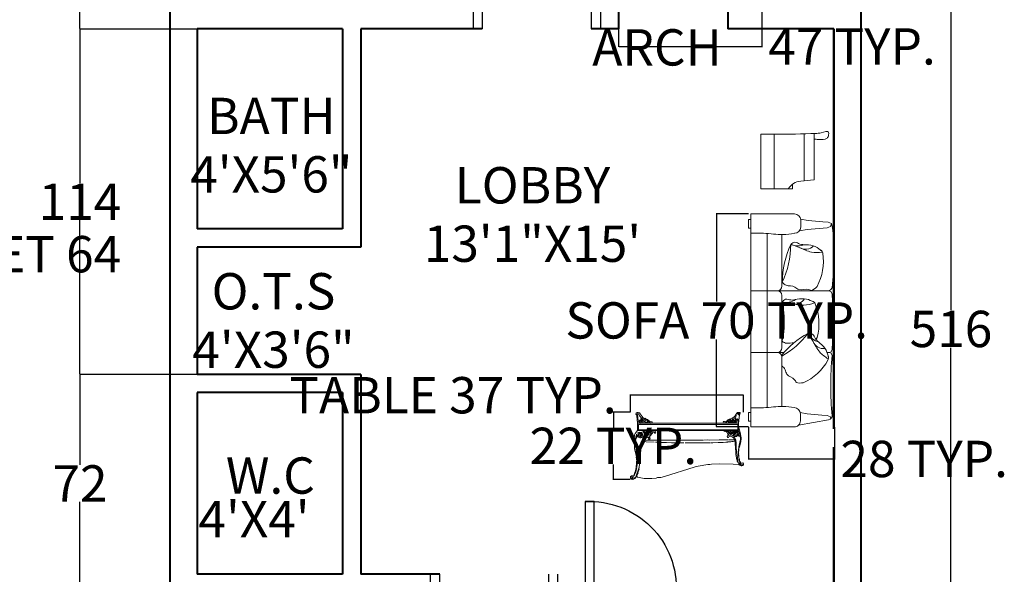
# Model space of a CAD drawing. Units: inches. Extents: x -124 to 612, y -69 to 524.
# Tile 8 of 9: x 287 to 612, y 146 to 329. Entities that reach past the tile are written whole.
import ezdxf
from ezdxf.enums import TextEntityAlignment as Align

# ---------------------------------------------------------------- set-up
doc = ezdxf.new("R2010")
doc.units = ezdxf.units.IN
doc.header["$MEASUREMENT"] = 0
for name, color, linetype, lineweight in [('A-ANNO-DIMS', 2, 'Continuous', 18), ('A-ANNO-TEXT', 1, 'Continuous', 18), ('A-AREA-IDEN', 1, 'Continuous', 18), ('A-DOOR', 4, 'Continuous', 25), ('A-FURN', 8, 'Continuous', 18), ('A-WALL', 7, 'Continuous', 40)]:
    doc.layers.add(name, color=color, linetype=linetype, lineweight=lineweight)
doc.styles.get("Standard").update_dxf_attribs({"font": 'arial.ttf'})
doc.dimstyles.get("Standard").update_dxf_attribs({"dimtxt": 12, "dimasz": 0.18, "dimexe": 0.18, "dimexo": 0.0625, "dimgap": 0.09, "dimtad": 0, "dimtih": 1, "dimtoh": 1, "dimdec": 0, "dimzin": 0, "dimdsep": 46, "dimlunit": 4, "dimtxsty": 'Standard', "dimcen": 0.09, "dimadec": 0, "dimazin": 0, "dimtfac": 1, "dimtdec": 0, "dimtofl": 0, "dimtmove": 0, "dimatfit": 3, "dimfxl": 1, "dimtolj": 1, "dimtzin": 0, "dimarcsym": 0})

# ---------------------------------------------------------------- blocks, each defined once
blk = doc.blocks.new('A$C32C86113')
for p, q in [((77.9, 721.3, -9.2), (82, 773.3, -9.2)), ((82, 773.3, -9.2), (93.6, 803.8, -9.2)), ((93.6, 803.8, -9.2), (123, 812.9, -9.2)), ((736.9, 798.3, -9.2), (719.4, 811.4, -9.2)), ((747.8, 782.5, -9.2), (736.9, 798.3, -9.2)), ((747.6, 163.7, -9.2), (747.6, 782.8, -9.2)), ((747.7, 782.8, -9.2), (758.8, 802, -9.2)), ((758.8, 802, -9.2), (780.7, 812.4, -9.2)), ((1340.4, 800.9, -9.2), (1318.5, 811.4, -9.2)), ((1347.6, 787, -9.2), (1340.4, 800.9, -9.2)), ((1347.6, 787, -9.2), (1354.9, 800.9, -9.2)), ((1347.6, 787, -9.2), (1347.6, 761.5, -9.2)), ((1354.9, 800.9, -9.2), (1376.9, 811.5, -9.2)), ((2056, 484.9, -9.2), (2002, 776.1, -9.2)), ((65.8, 577.5, -9.2), (77.9, 721.3, -9.2)), ((51.2, 502.4, -9.2), (65.8, 577.5, -9.2)), ((60.2, 506.2, -9.2), (128.9, 506.2, -9.2)), ((2013.7, 502.6, -9.2), (1944.9, 502.8, -9.2)), ((0.2, 446.2, -9.2), (0, 20, -9.2)), ((2071.8, 20, 333.6), (2071.8, 442.4, 333.6)), ((702.6, 323.7, -9.2), (200, 323.4, -0.7)), ((1302.6, 323.7, -9.2), (792.6, 323.7, -9.2)), ((1347.6, 343.7, -9.2), (1347.6, 278.7, -9.2)), ((1872.8, 323.7, -9.2), (1392.6, 323.7, -9.2)), ((747.6, 20, -9.2), (747.6, 278.7, -9.2)), ((1347.6, 278.7, -9.2), (1347.6, 20, -9.2)), ((2071.8, 20, 333.6), (0, 20, -9.2)), ((55.9, 20), (55.9, 0)), ((139, 0), (139, 20, 13.8)), ((1932.8, 0), (1932.8, 20, 13.8)), ((2015.9, 20), (2015.9, 0)), ((55.9, 0), (139, 0)), ((2015.9, 0), (1932.8, 0))]:
    blk.add_line(p, q)
at = {"ltscale": 3}
for p, q in [((123, 794.8, -9.2), (93.6, 803.8, -9.2)), ((134.6, 764.2, -9.2), (123, 794.8, -9.2)), ((1960.7, 764.2, -9.2), (1972.3, 794.8, -9.2)), ((1972.3, 794.8, -9.2), (1989.3, 800, -9.2)), ((150.8, 568.4, -9.2), (134.6, 764.2, -9.2)), ((1944.5, 568.4, -9.2), (1956.6, 712.2, -9.2)), ((1956.6, 712.2, -9.2), (1960.7, 764.2, -9.2)), ((165.4, 493.4, -9.2), (150.8, 568.4, -9.2)), ((1931.4, 501.4, -9.2), (1944.5, 568.4, -9.2)), ((191.4, 179.1, 242), (1883, 179.1, 242))]:
    blk.add_line(p, q, dxfattribs=at)
for centre, radius, start, end in [((414.4, -1890.5, -9.2), 2719, 83.56046, 96.1533), ((1675, -2302.2, -9.2), 3127.9, 84.6632, 95.46976), ((1399.9, 730.9, 333.6), 45, 61.39238, 113.21883), ((1178.3, 324.5, 333.6), 507.8, 23.79865, 61.39238), ((1957.7, 767.9, -9.2), 45, 10.50914, 90), ((390.8, 676.1, 333.6), 45, 98.91064, 150.73708), ((462.5, 218.9, 333.6), 507.8, 61.3169, 98.91064), ((1065.4, 175.7, 333.6), 507.8, 74.38291, 111.97665), ((594.5, 543.8, 333.6), 164.4, 23.69861, 47.17942), ((892.1, 605, 333.6), 45, 111.97665, 163.80309), ((1917, 985.8, 333.6), 858.1, 208.49339, 231.11555), ((1120.5, 522.1, 333.6), 164.4, 52.76952, 60.24543), ((60.2, 446.2, -9.2), 60, 90, 179.98162), ((128.9, 446.2, -9.2), 60, 0, 90), ((1480.8, 501.9, 333.6), 164.4, 346.18035, 9.66116), ((1944.7, 442.8, -9.2), 60, 89.78593, 179.78593), ((2014.6, 445.3, 333.6), 57.3, 357.05812, 90.92062), ((691.5, 1297, 333.6), 971.5, 246.03307, 268.4688), ((702.6, 278.7, -9.2), 45, 0, 90), ((792.6, 278.7, -9.2), 45, 90, 180), ((1054.6, -512.3, 333.6), 858.1, 76.95935, 103.04065), ((1302.6, 278.7, -9.2), 45, 0, 90), ((1392.6, 278.7, -9.2), 45, 90, 180)]:
    blk.add_arc(centre, radius, start, end)
for centre, radius, start, end in [((1034.7, -7187.9, -9.2), 8004.3, 87.96784, 91.81809), ((1675, 3925.1, -9.2), 3127.9, 264.53024, 275.3368), ((1072.8, 736, 333.6), 183.2, 299.4203, 342.7126), ((1202.4, 727.4, 333.6), 108.4, 291.46137, 8.04974), ((236.2, 553.1, 333.6), 108.4, 328.97962, 45.56799), ((639.9, -104, 333.6), 858.1, 29.83423, 52.45639), ((128.3, 481, 333.6), 183.2, 336.93856, 20.23086), ((769.4, 450.2, 333.6), 108.4, 342.04563, 58.634), ((296.4, -448.9, 333.6), 858.1, 64.52723, 89.97465), ((680.5, 355.5, 333.6), 183.2, 350.00456, 33.29687)]:
    blk.add_arc(centre, radius, start, end, dxfattribs=at)
for points, knots in [([(1402, 775.8, 333.6), (1375.6, 770, 333.6), (1319.1, 757.7, 333.6), (1261.1, 701.8, 333.6), (1222.2, 646.1, 333.6), (1162.2, 629.7, 333.6), (1162.6, 593.5, 333.6), (1162.8, 576.4, 333.6)], [0, 0, 0, 0, 79.746539, 170.719486, 232.023986, 283.143815, 329.425672, 329.425672, 329.425672, 329.425672]), ([(365.1, 713.1, 333.6), (347.7, 692.4, 333.6), (310.4, 648.2, 333.6), (298.4, 568.5, 333.6), (301.5, 500.7, 333.6), (263.9, 451.1, 333.6), (286.2, 422.7, 333.6), (296.8, 409.2, 333.6)], [0, 0, 0, 0, 79.746539, 170.719486, 232.023986, 283.143815, 329.425672, 329.425672, 329.425672, 329.425672]), ([(745, 609.9, 333.6), (745, 609.9, 333.6), (718.2, 560.7, 333.6), (755.5, 498.7, 333.6), (695.1, 438.3, 333.6), (705.8, 371.4, 333.6), (679.8, 337.8, 333.6), (665.5, 325.8, 333.6)], [27.786417, 27.786417, 27.786417, 27.786417, 60.334214, 153.42843, 198.910048, 289.238615, 341.466319, 341.466319, 341.466319, 341.466319]), ([(858.8, 635.1, 333.6), (846.5, 611.1, 333.6), (820.1, 559.5, 333.6), (826.5, 479.3, 333.6), (844.8, 413.9, 333.6), (819.4, 357.1, 333.6), (847.6, 334.4, 333.6), (860.9, 323.7, 333.6)], [0, 0, 0, 0, 79.746539, 170.719486, 232.023986, 283.143815, 329.425672, 329.425672, 329.425672, 329.425672]), ([(189.7, 443.1, -9.2), (195.9, 408.3, 46.7), (209, 335.3, 164.5), (187, 169.8, 251), (187.5, 61.2, 288.7), (187.7, 20, 303)], [0, 0, 0, 0, 194.838243, 409.817627, 541.189597, 541.189597, 541.189597, 541.189597]), ([(1253.9, 441, 333.6), (1252.3, 416.7, 333.6), (1266, 375.1, 333.6), (1250.1, 340.7, 333.6), (1238.9, 325.8, 333.6)], [214.332348, 214.332348, 214.332348, 214.332348, 289.238615, 341.466319, 341.466319, 341.466319, 341.466319]), ([(1640.5, 462.6, 333.6), (1640.5, 462.6, 333.6), (1589.2, 439.9, 333.6), (1581.1, 368, 333.6), (1510.9, 358.8, 333.6), (1488.8, 335.7, 333.6), (1477.6, 323.7, 333.6)], [27.786417, 27.786417, 27.786417, 27.786417, 60.334214, 153.42843, 198.910048, 250.027656, 250.027656, 250.027656, 250.027656]), ([(1884.7, 443.1, -9.2), (1878.5, 408.3, 46.7), (1865.4, 335.3, 164.5), (1887.4, 169.8, 251), (1886.9, 61.2, 288.7), (1886.7, 20, 303)], [0, 0, 0, 0, 194.838243, 409.817627, 541.189597, 541.189597, 541.189597, 541.189597])]:
    blk.add_open_spline(points, degree=3, knots=knots)
for points in [[(1409.2, 771.8, 333.6), (1389.5, 742.5, 333.6), (1346.6, 678.6, 333.6), (1247.3, 632.8, 333.6), (1188.1, 593.3, 333.6), (1162.8, 576.4, 333.6)], [(373.3, 714.3, 333.6), (375.5, 679, 333.6), (380.4, 602.2, 333.6), (329.5, 505.4, 333.6), (306.6, 438, 333.6), (296.8, 409.2, 333.6)], [(866.4, 638.2, 333.6), (876.6, 604.3, 333.6), (898.7, 530.5, 333.6), (871, 424.8, 333.6), (864, 353.9, 333.6), (860.9, 323.7, 333.6)]]:
    blk.add_open_spline(points, degree=3, knots=[0, 0, 0, 0, 104.254828, 226.968516, 318.497377, 318.497377, 318.497377, 318.497377], dxfattribs=at)
blk = doc.blocks.new('A$C43184A5C')
for p, q in [((724, 800), (30, 800)), ((724, 795), (724, 800)), ((740, 650), (35, 650)), ((856, 474), (788, 474)), ((856, 0), (856, 474)), ((856, 200), (42, 200)), ((856, 0), (39, 0)), ((39, 0), (39, 0))]:
    blk.add_line(p, q)
for points, knots in [([(116, 800), (117, 819), (120, 882), (131, 984), (59, 1017), (-22, 1023), (26, 905), (34, 661), (46, 339), (41, 68), (39, 0)], [4.965253, 4.965253, 4.965253, 4.965253, 63.558713, 198.678228, 250.994518, 291.108293, 401.549508, 488.981253, 1103.790728, 1307.592638, 1307.592638, 1307.592638, 1307.592638]), ([(855, 414), (825, 437), (765, 483), (737, 627), (729, 730), (724, 795)], [0, 0, 0, 0, 106.359769, 221.555283, 419.666547, 419.666547, 419.666547, 419.666547])]:
    blk.add_open_spline(points, degree=3, knots=knots)
blk = doc.blocks.new('A$C0D2616A3')
for p, q in [((673, 750), (1080, 882)), ((1080, 882), (1131, 892)), ((1131, 892), (1176, 896)), ((1176, 896), (1194, 901)), ((1194, 901), (1255, 907)), ((1255, 907), (1361, 907)), ((1361, 907), (1451, 890)), ((1429, 761), (1459, 868)), ((1430, 752), (1481, 898)), ((1431, 780), (1442, 814)), ((1444, 829), (1452, 852)), ((1449, 818), (1461, 845)), ((1451, 890), (1463, 882)), ((1455, 859), (1463, 875)), ((1474, 891), (1463, 875)), ((1467, 781), (1480, 828)), ((1471, 803), (1482, 837)), ((1483, 893), (1474, 891)), ((1479, 889), (1474, 891)), ((1478, 893), (1479, 889)), ((1481, 898), (1490, 907)), ((1483, 896), (1481, 898)), ((1482, 833), (1488, 844)), ((1494, 905), (1483, 896)), ((1488, 849), (1502, 871)), ((1493, 844), (1488, 849)), ((1503, 910), (1490, 907)), ((1491, 851), (1504, 862)), ((1498, 909), (1512, 914)), ((1502, 871), (1508, 872)), ((1530, 912), (1503, 910)), ((1506, 865), (1510, 896)), ((1508, 872), (1517, 869)), ((1510, 896), (1516, 903)), ((1516, 903), (1523, 903)), ((1517, 869), (1535, 870)), ((1526, 897), (1521, 892)), ((1521, 892), (1524, 885)), ((1523, 903), (1526, 897)), ((1524, 885), (1535, 886)), ((1537, 904), (1530, 912)), ((9, 695), (16, 693)), ((24, 724), (14, 717)), ((16, 693), (28, 699)), ((40, 718), (24, 724)), ((30, 700), (34, 704)), ((37, 691), (30, 700)), ((34, 704), (36, 715)), ((41, 698), (36, 704)), ((45, 691), (37, 691)), ((57, 702), (40, 718)), ((41, 684), (41, 698)), ((48, 675), (41, 684)), ((53, 680), (45, 691)), ((48, 671), (53, 680)), ((68, 694), (56, 720)), ((63, 703), (57, 702)), ((58, 720), (61, 721)), ((61, 721), (140, 709)), ((97, 514), (70, 693)), ((70, 693), (73, 692)), ((73, 692), (92, 642)), ((84, 671), (79, 682)), ((140, 709), (324, 706)), ((324, 706), (439, 709)), ((439, 709), (460, 715)), ((1409, 543), (1430, 755)), ((1420, 656), (1423, 726)), ((1422, 705), (1428, 710)), ((1423, 726), (1428, 743)), ((1452, 679), (1453, 703)), ((1452, 674), (1452, 679)), ((1453, 703), (1455, 712)), ((1455, 712), (1461, 758)), ((1463, 765), (1465, 776)), ((1465, 776), (1467, 781)), ((53, 668), (54, 644)), ((54, 644), (63, 637)), ((60, 660), (55, 671)), ((61, 592), (60, 660)), ((63, 630), (61, 628)), ((61, 596), (65, 626)), ((66, 587), (61, 592)), ((62, 570), (66, 576)), ((67, 565), (62, 570)), ((65, 626), (63, 630)), ((68, 506), (66, 599)), ((82, 651), (78, 664)), ((97, 622), (85, 664)), ((96, 627), (94, 636)), ((102, 580), (97, 622)), ((104, 575), (102, 580)), ((104, 568), (104, 575)), ((105, 561), (104, 568)), ((105, 537), (105, 561)), ((1409, 538), (1409, 543)), ((1413, 473), (1424, 611)), ((1423, 653), (1420, 656)), ((1424, 611), (1421, 619)), ((1452, 645), (1452, 674)), ((1453, 636), (1452, 645)), ((1453, 623), (1453, 636)), ((1455, 618), (1453, 623)), ((1455, 611), (1455, 618)), ((1463, 580), (1455, 611)), ((1469, 612), (1463, 670)), ((1465, 564), (1463, 578)), ((1468, 549), (1465, 564)), ((1468, 544), (1466, 555)), ((1471, 526), (1468, 544)), ((30, 359), (36, 405)), ((36, 405), (42, 416)), ((42, 416), (55, 479)), ((43, 386), (62, 471)), ((55, 479), (61, 497)), ((63, 527), (67, 533)), ((64, 475), (63, 527)), ((65, 502), (68, 506)), ((99, 509), (97, 514)), ((98, 467), (99, 503)), ((99, 433), (98, 467)), ((99, 503), (99, 509)), ((101, 428), (99, 433)), ((106, 383), (101, 422)), ((106, 530), (105, 537)), ((106, 516), (106, 530)), ((108, 508), (106, 516)), ((108, 494), (108, 508)), ((109, 481), (108, 494)), ((112, 435), (109, 481)), ((114, 427), (112, 435)), ((114, 422), (118, 382)), ((185, 405), (191, 406)), ((212, 406), (191, 406)), ((212, 406), (219, 408)), ((227, 407), (219, 408)), ((227, 407), (237, 409)), ((243, 409), (237, 409)), ((243, 409), (279, 412)), ((293, 412), (279, 412)), ((293, 412), (315, 413)), ((327, 413), (315, 413)), ((327, 413), (336, 415)), ((344, 414), (336, 415)), ((344, 414), (417, 417)), ((430, 417), (417, 417)), ((448, 416), (430, 417)), ((457, 418), (506, 419)), ((511, 419), (506, 419)), ((511, 419), (585, 419)), ((592, 419), (585, 419)), ((666, 418), (592, 419)), ((666, 418), (685, 419)), ((745, 418), (685, 419)), ((759, 418), (745, 418)), ((772, 418), (759, 418)), ((799, 417), (772, 418)), ((817, 417), (977, 416)), ((984, 416), (977, 416)), ((1052, 413), (984, 416)), ((1124, 412), (1057, 413)), ((1144, 409), (1138, 410)), ((1178, 411), (1153, 411)), ((1203, 408), (1185, 409)), ((1332, 404), (1223, 408)), ((1392, 411), (1398, 436)), ((1393, 393), (1411, 468)), ((1398, 436), (1400, 441)), ((1400, 441), (1402, 459)), ((1402, 459), (1404, 475)), ((1406, 482), (1404, 470)), ((1411, 488), (1406, 482)), ((1409, 538), (1408, 533)), ((1408, 533), (1408, 491)), ((1408, 491), (1411, 488)), ((1411, 468), (1413, 473)), ((1471, 519), (1471, 526)), ((1473, 504), (1471, 519)), ((1472, 494), (1473, 504)), ((1474, 486), (1472, 494)), ((1474, 468), (1474, 486)), ((1476, 461), (1474, 468)), ((1475, 450), (1476, 461)), ((1477, 434), (1475, 450)), ((1476, 404), (1477, 423)), ((1477, 423), (1477, 434)), ((34, 316), (30, 359)), ((40, 310), (34, 316)), ((39, 294), (41, 380)), ((51, 259), (39, 294)), ((42, 332), (45, 335)), ((50, 288), (43, 299)), ((71, 257), (43, 290)), ((45, 335), (54, 322)), ((46, 285), (48, 292)), ((54, 322), (56, 315)), ((58, 310), (71, 327)), ((59, 288), (58, 310)), ((69, 322), (70, 313)), ((70, 313), (70, 288)), ((96, 331), (72, 313)), ((81, 297), (85, 306)), ((82, 288), (81, 297)), ((116, 332), (96, 331)), ((104, 300), (108, 293)), ((118, 350), (106, 383)), ((132, 328), (107, 379)), ((107, 266), (116, 275)), ((112, 253), (143, 281)), ((120, 269), (115, 271)), ((160, 312), (116, 332)), ((118, 391), (135, 398)), ((118, 382), (124, 377)), ((129, 278), (120, 269)), ((124, 377), (123, 368)), ((124, 395), (147, 402)), ((125, 377), (152, 378)), ((136, 348), (127, 361)), ((129, 303), (131, 281)), ((154, 272), (134, 254)), ((145, 287), (135, 325)), ((143, 281), (176, 306)), ((158, 401), (147, 402)), ((152, 378), (190, 379)), ((178, 288), (156, 276)), ((158, 401), (174, 405)), ((198, 307), (160, 312)), ((167, 284), (170, 259)), ((185, 405), (174, 405)), ((177, 264), (179, 272)), ((192, 279), (178, 288)), ((179, 272), (192, 271)), ((196, 291), (181, 290)), ((197, 379), (190, 379)), ((192, 271), (192, 279)), ((196, 327), (206, 343)), ((205, 282), (196, 291)), ((198, 309), (218, 323)), ((217, 294), (198, 307)), ((202, 250), (226, 273)), ((206, 266), (205, 282)), ((239, 378), (206, 379)), ((206, 343), (216, 345)), ((216, 345), (220, 341)), ((223, 278), (217, 294)), ((220, 341), (222, 328)), ((226, 273), (240, 262)), ((244, 378), (285, 379)), ((305, 379), (285, 379)), ((311, 379), (305, 379)), ((320, 379), (311, 379)), ((325, 379), (320, 379)), ((334, 379), (325, 379)), ((334, 379), (471, 380)), ((494, 379), (471, 380)), ((494, 379), (544, 380)), ((557, 380), (552, 380)), ((557, 380), (708, 381)), ((769, 380), (708, 381)), ((769, 380), (794, 381)), ((802, 381), (794, 381)), ((802, 381), (906, 381)), ((917, 381), (900, 381)), ((917, 381), (976, 382)), ((1008, 381), (976, 382)), ((1008, 381), (1044, 382)), ((1095, 382), (1044, 382)), ((1095, 382), (1118, 383)), ((1141, 383), (1118, 383)), ((1147, 382), (1141, 383)), ((1158, 382), (1147, 382)), ((1158, 382), (1237, 383)), ((1201, 272), (1204, 279)), ((1204, 279), (1208, 284)), ((1208, 284), (1217, 284)), ((1217, 284), (1217, 266)), ((1219, 266), (1217, 279)), ((1233, 266), (1262, 299)), ((1269, 382), (1237, 383)), ((1240, 250), (1264, 274)), ((1262, 299), (1266, 308)), ((1264, 276), (1262, 296)), ((1264, 274), (1279, 251)), ((1266, 308), (1268, 314)), ((1268, 314), (1272, 319)), ((1282, 382), (1269, 382)), ((1272, 319), (1288, 335)), ((1273, 285), (1279, 303)), ((1280, 269), (1273, 285)), ((1287, 261), (1275, 279)), ((1281, 366), (1279, 353)), ((1279, 353), (1292, 339)), ((1279, 303), (1288, 312)), ((1287, 373), (1281, 366)), ((1289, 382), (1282, 382)), ((1292, 339), (1283, 332)), ((1289, 382), (1296, 383)), ((1297, 313), (1291, 313)), ((1291, 281), (1293, 294)), ((1294, 277), (1291, 281)), ((1303, 349), (1294, 356)), ((1294, 339), (1331, 332)), ((1298, 275), (1294, 277)), ((1320, 383), (1296, 383)), ((1297, 313), (1302, 315)), ((1320, 298), (1298, 299)), ((1302, 286), (1298, 275)), ((1325, 307), (1302, 315)), ((1309, 290), (1302, 286)), ((1319, 347), (1303, 349)), ((1314, 284), (1309, 290)), ((1316, 268), (1314, 284)), ((1366, 370), (1319, 347)), ((1381, 389), (1320, 383)), ((1329, 288), (1320, 298)), ((1331, 302), (1325, 307)), ((1326, 261), (1330, 271)), ((1330, 271), (1329, 288)), ((1330, 350), (1346, 356)), ((1331, 332), (1356, 309)), ((1371, 247), (1331, 302)), ((1361, 402), (1332, 404)), ((1333, 334), (1364, 346)), ((1350, 273), (1338, 293)), ((1342, 338), (1353, 341)), ((1359, 291), (1362, 319)), ((1368, 265), (1359, 291)), ((1384, 341), (1362, 319)), ((1380, 252), (1363, 278)), ((1372, 377), (1370, 382)), ((1388, 281), (1383, 301)), ((1400, 347), (1384, 341)), ((1385, 315), (1409, 335)), ((1385, 296), (1385, 315)), ((1400, 270), (1388, 281)), ((1391, 344), (1407, 347)), ((1427, 270), (1393, 276)), ((1396, 308), (1395, 290)), ((1395, 290), (1408, 279)), ((1405, 320), (1396, 308)), ((1400, 333), (1407, 335)), ((1412, 322), (1405, 320)), ((1406, 304), (1419, 311)), ((1408, 293), (1406, 304)), ((1407, 347), (1412, 349)), ((1415, 290), (1408, 293)), ((1408, 279), (1427, 279)), ((1420, 349), (1412, 349)), ((1419, 315), (1412, 322)), ((1420, 290), (1415, 290)), ((1419, 311), (1419, 315)), ((1427, 347), (1420, 349)), ((1428, 295), (1420, 290)), ((1426, 293), (1431, 306)), ((1427, 347), (1430, 347)), ((1455, 287), (1427, 270)), ((1427, 279), (1433, 284)), ((1430, 300), (1428, 295)), ((1430, 347), (1453, 327)), ((1433, 284), (1444, 309)), ((1438, 291), (1442, 302)), ((1444, 329), (1448, 334)), ((1446, 323), (1444, 329)), ((1444, 309), (1446, 323)), ((1453, 327), (1472, 352)), ((1454, 249), (1485, 290)), ((1455, 309), (1455, 325)), ((1459, 332), (1466, 348)), ((1466, 301), (1471, 326)), ((1473, 330), (1476, 366)), ((1476, 366), (1478, 373)), ((1478, 393), (1478, 398)), ((1478, 387), (1478, 393)), ((1478, 373), (1478, 387)), ((1487, 294), (1495, 315)), ((70, 175), (51, 259)), ((65, 119), (67, 144)), ((67, 248), (1452, 248)), ((67, 150), (67, 248)), ((1452, 150), (67, 150)), ((111, 249), (71, 257)), ((74, 137), (71, 149)), ((76, 115), (74, 137)), ((78, 240), (1439, 240)), ((78, 166), (78, 240)), ((1439, 166), (78, 166)), ((89, 124), (107, 147)), ((119, 136), (108, 127)), ((136, 136), (119, 136)), ((146, 121), (136, 136)), ((157, 126), (138, 150)), ((161, 137), (159, 146)), ((173, 140), (166, 150)), ((170, 259), (177, 250)), ((186, 255), (177, 264)), ((197, 140), (186, 144)), ((190, 253), (204, 262)), ((202, 135), (197, 140)), ((211, 140), (213, 127)), ((214, 111), (247, 150)), ((238, 249), (222, 265)), ((240, 262), (255, 260)), ((255, 260), (262, 265)), ((262, 265), (265, 261)), ((265, 261), (265, 254)), ((276, 133), (272, 146)), ((1199, 268), (1211, 250)), ((1217, 266), (1233, 266)), ((1250, 132), (1251, 150)), ((1315, 106), (1272, 152)), ((1303, 257), (1287, 261)), ((1312, 264), (1303, 257)), ((1308, 144), (1306, 128)), ((1317, 252), (1326, 261)), ((1320, 122), (1321, 137)), ((1348, 143), (1348, 138)), ((1348, 138), (1353, 131)), ((1369, 125), (1385, 143)), ((1398, 142), (1382, 141)), ((1407, 135), (1398, 142)), ((1409, 151), (1439, 118)), ((1439, 240), (1439, 166)), ((1439, 118), (1445, 136)), ((1445, 136), (1448, 143)), ((1452, 248), (1452, 150)), ((1455, 104), (1454, 150)), ((81, 4), (50, 1)), ((53, 33), (61, 110)), ((67, 34), (55, 33)), ((60, 18), (71, 31)), ((60, 13), (60, 18)), ((70, 4), (60, 13)), ((61, 110), (65, 119)), ((81, 90), (65, 112)), ((71, 31), (67, 34)), ((69, 7), (83, 25)), ((86, 104), (78, 112)), ((86, 95), (81, 90)), ((107, 34), (81, 4)), ((99, 120), (86, 95)), ((93, 45), (122, 68)), ((99, 120), (108, 127)), ((101, 99), (103, 104)), ((102, 82), (101, 99)), ((115, 70), (102, 82)), ((103, 104), (105, 111)), ((105, 111), (112, 120)), ((109, 37), (112, 46)), ((112, 120), (128, 123)), ((112, 46), (127, 62)), ((120, 86), (135, 87)), ((122, 68), (125, 64)), ((127, 62), (156, 81)), ((128, 123), (137, 118)), ((135, 87), (146, 98)), ((146, 98), (146, 121)), ((156, 85), (157, 126)), ((156, 81), (160, 80)), ((160, 80), (172, 83)), ((182, 94), (174, 87)), ((189, 93), (182, 94)), ((247, 130), (192, 95)), ((193, 119), (202, 127)), ((204, 117), (193, 119)), ((202, 106), (194, 101)), ((202, 127), (202, 135)), ((210, 100), (202, 106)), ((211, 124), (204, 117)), ((218, 104), (207, 108)), ((211, 109), (210, 100)), ((258, 132), (247, 130)), ((263, 126), (258, 132)), ((272, 126), (263, 126)), ((276, 130), (272, 126)), ((1254, 129), (1250, 132)), ((1279, 130), (1254, 129)), ((1315, 97), (1279, 130)), ((1306, 128), (1313, 122)), ((1313, 122), (1320, 122)), ((1327, 106), (1315, 106)), ((1338, 99), (1315, 97)), ((1336, 113), (1327, 106)), ((1345, 80), (1334, 95)), ((1340, 124), (1339, 135)), ((1340, 102), (1347, 107)), ((1358, 89), (1345, 80)), ((1351, 111), (1347, 98)), ((1358, 96), (1351, 111)), ((1353, 114), (1360, 134)), ((1375, 76), (1358, 89)), ((1373, 134), (1370, 98)), ((1416, 22), (1375, 76)), ((1381, 114), (1394, 126)), ((1381, 105), (1381, 114)), ((1385, 101), (1381, 105)), ((1382, 73), (1397, 78)), ((1390, 101), (1385, 101)), ((1397, 110), (1390, 101)), ((1394, 126), (1398, 126)), ((1405, 106), (1397, 110)), ((1407, 117), (1398, 126)), ((1408, 88), (1399, 78)), ((1399, 78), (1420, 54)), ((1403, 123), (1410, 113)), ((1410, 113), (1408, 88)), ((1428, 106), (1410, 131)), ((1423, 49), (1416, 59)), ((1423, 49), (1441, 14)), ((1432, 25), (1427, 38)), ((1446, 102), (1428, 106)), ((1441, 120), (1445, 129)), ((1441, 14), (1453, 14)), ((1445, 77), (1446, 86)), ((1445, 66), (1445, 77)), ((1452, 44), (1445, 66)), ((1446, 86), (1446, 102)), ((1456, 41), (1450, 48)), ((1454, 39), (1450, 35)), ((1450, 35), (1455, 19)), ((1459, 48), (1455, 104)), ((1459, 42), (1456, 41)), ((1463, 39), (1475, 26)), ((1475, 26), (1475, 15))]:
    blk.add_line(p, q)
for centre, radius, start, end in [((1915, 682), 450, 158.9779, 181.5094), ((1519, 892), 28.8, 305.8699, 146.9946), ((21, 711), 21.6, 93.3987, 231.125), ((25, 693), 39.6, 40.4237, 96.4314), ((379, 1827), 1115, 274.1777, 285.275), ((746, 397), 752, 353.7932, 16.6146), ((100, 293), 28.8, 189.008, 283.9314), ((97, 287), 10.8, 179, 25.5651), ((108, 293), 23.4, 25.5651, 150.6992), ((108, 287), 12.6, 319.1944, 104.9454), ((183, 385), 59.3, 195.8584, 283.0362), ((1292, 364), 7.19, 283.0362, 119.9638), ((1414, 311), 21.6, 342.3008, 106.1027), ((196, 118), 27, 124.5377, 234.3048), ((211, 125), 30.6, 136.1211, 249.56), ((1330, 133), 8.99, 10.3099, 157.1986), ((63, 15), 18, 119.9638, 227.8141), ((126, 98), 14.4, 103.0362, 245.8014), ((135, 111), 7.19, 170.8699, 74.9638), ((1388, 103), 16.2, 195.6992, 11.5288), ((1446, 32), 32.4, 198.44, 322.7462)]:
    blk.add_arc(centre, radius, start, end)
blk = doc.blocks.new('DOOR-36IN-SINGLE')
for p, q in [((0, 6), (0, 0)), ((3, 6), (3, 0)), ((39, 6), (39, 0)), ((42, 6), (42, 0))]:
    blk.add_line(p, q)
blk.add_lwpolyline([(39, 6), (36, 6), (36, 42), (39, 42)], close=True)
blk.add_arc((37.5, 7.5), 34.53, 87.5104, 182.4896)
blk = doc.blocks.new('DOOR-30IN-STAIR')
for p, q in [((0, 30.04), (0, 36.04)), ((3, 30.04), (3, 36.04)), ((33, 30.04), (33, 36.04)), ((36, 30.04), (36, 36.04))]:
    blk.add_line(p, q)
blk.add_lwpolyline([(3, 30.04), (6, 30.04), (6, 0.04), (3, 0.04)], close=True)
blk.add_arc((4.5, 28.54), 28.54, 266.9872, 3.0128)
blk = doc.blocks.new('*D25')
at = {"layer": 'A-ANNO-DIMS', "color": 0, "lineweight": -2, "transparency": 16777216}
for p, q in [((527.87, 265.09), (517.2, 265.09)), ((517.38, 264.91), (517.38, 236.21)), ((517.38, 194.92), (517.38, 223.61)), ((527.87, 194.74), (517.2, 194.74))]:
    blk.add_line(p, q, dxfattribs=at)
at = {"layer": 'A-ANNO-DIMS', "color": 0, "transparency": 16777216}
for points in [[(517.35, 264.91), (517.41, 264.91), (517.38, 265.09)], [(517.35, 194.92), (517.41, 194.92), (517.38, 194.74)]]:
    blk.add_solid(points, dxfattribs=at)
at = {"layer": 'Defpoints', "color": 0, "transparency": 16777216}
for p in [(527.93, 265.09), (517.38, 194.74), (527.93, 194.74)]:
    blk.add_point(p, dxfattribs=at)
at = {"layer": 'A-ANNO-DIMS', "color": 0, "transparency": 16777216, "insert": (517.38, 229.91), "char_height": 12, "attachment_point": 5}
blk.add_mtext('\\A1;SOFA 70 TYP.', dxfattribs=at)
blk = doc.blocks.new('*D26')
at = {"layer": 'A-ANNO-DIMS', "color": 0, "lineweight": -2, "transparency": 16777216}
for p, q in [((527.93, 194.68), (527.93, 184.01)), ((556.25, 194.68), (556.25, 184.01)), ((528.11, 184.19), (556.07, 184.19)), ((556.25, 184.19), (556.43, 184.19))]:
    blk.add_line(p, q, dxfattribs=at)
at = {"layer": 'A-ANNO-DIMS', "color": 0, "transparency": 16777216}
for points in [[(528.11, 184.22), (528.11, 184.16), (527.93, 184.19)], [(556.07, 184.22), (556.07, 184.16), (556.25, 184.19)]]:
    blk.add_solid(points, dxfattribs=at)
at = {"layer": 'Defpoints', "color": 0, "transparency": 16777216}
for p in [(527.93, 194.74), (556.25, 194.74), (556.25, 184.19)]:
    blk.add_point(p, dxfattribs=at)
at = {"layer": 'A-ANNO-DIMS', "color": 0, "transparency": 16777216, "insert": (585.83, 184.19), "char_height": 12, "attachment_point": 5}
blk.add_mtext('\\A1;28 TYP.', dxfattribs=at)
blk = doc.blocks.new('*D29')
at = {"layer": 'A-ANNO-DIMS', "color": 0, "lineweight": -2, "transparency": 16777216}
for p, q in [((488.91, 205.22), (488.73, 205.22)), ((488.91, 199.68), (488.91, 205.4)), ((526.07, 205.22), (489.09, 205.22)), ((526.25, 199.68), (526.25, 205.4))]:
    blk.add_line(p, q, dxfattribs=at)
at = {"layer": 'A-ANNO-DIMS', "color": 0, "transparency": 16777216}
for points in [[(489.09, 205.25), (489.09, 205.19), (488.91, 205.22)], [(526.07, 205.25), (526.07, 205.19), (526.25, 205.22)]]:
    blk.add_solid(points, dxfattribs=at)
at = {"layer": 'Defpoints', "color": 0, "transparency": 16777216}
for p in [(488.91, 205.22), (488.91, 199.62), (526.25, 199.62)]:
    blk.add_point(p, dxfattribs=at)
at = {"layer": 'A-ANNO-DIMS', "color": 0, "transparency": 16777216, "insert": (430.4, 205.22), "char_height": 12, "attachment_point": 5}
blk.add_mtext('\\A1;TABLE 37 TYP.', dxfattribs=at)
blk = doc.blocks.new('*D30')
at = {"layer": 'A-ANNO-DIMS', "color": 0, "lineweight": -2, "transparency": 16777216}
for p, q in [((488.85, 199.62), (483.13, 199.62)), ((483.31, 199.44), (483.31, 194.62)), ((483.31, 177.55), (483.31, 182.38)), ((488.85, 177.37), (483.13, 177.37))]:
    blk.add_line(p, q, dxfattribs=at)
at = {"layer": 'A-ANNO-DIMS', "color": 0, "transparency": 16777216}
for points in [[(483.28, 199.44), (483.34, 199.44), (483.31, 199.62)], [(483.28, 177.55), (483.34, 177.55), (483.31, 177.37)]]:
    blk.add_solid(points, dxfattribs=at)
at = {"layer": 'Defpoints', "color": 0, "transparency": 16777216}
for p in [(488.91, 199.62), (483.31, 177.37), (488.91, 177.37)]:
    blk.add_point(p, dxfattribs=at)
at = {"layer": 'A-ANNO-DIMS', "color": 0, "transparency": 16777216, "insert": (483.31, 188.5), "char_height": 12, "attachment_point": 5}
blk.add_mtext('\\A1;22 TYP.', dxfattribs=at)
blk = doc.blocks.new('*D44')
at = {"layer": 'A-ANNO-DIMS', "color": 0, "lineweight": -2, "transparency": 16777216}
for p, q in [((485.02, 332.04), (485.02, 320.18)), ((532.32, 332.04), (532.32, 320.18)), ((485.2, 320.36), (532.14, 320.36)), ((532.32, 320.36), (532.5, 320.36))]:
    blk.add_line(p, q, dxfattribs=at)
at = {"layer": 'A-ANNO-DIMS', "color": 0, "transparency": 16777216}
for points in [[(485.2, 320.39), (485.2, 320.33), (485.02, 320.36)], [(532.14, 320.39), (532.14, 320.33), (532.32, 320.36)]]:
    blk.add_solid(points, dxfattribs=at)
at = {"layer": 'Defpoints', "color": 0, "transparency": 16777216}
for p in [(485.02, 332.1), (532.32, 332.1), (532.32, 320.36)]:
    blk.add_point(p, dxfattribs=at)
at = {"layer": 'A-ANNO-DIMS', "color": 0, "transparency": 16777216, "insert": (562.03, 320.36), "char_height": 12, "attachment_point": 5}
blk.add_mtext('\\A1;47 TYP.', dxfattribs=at)
blk = doc.blocks.new('*D45')
at = {"layer": 'A-ANNO-DIMS', "color": 0, "lineweight": -2, "transparency": 16777216}
for p, q in [((142.74, 261.33), (142.74, 251.59)), ((206.86, 261.33), (206.86, 251.59)), ((142.92, 251.77), (206.68, 251.77)), ((206.86, 251.77), (207.04, 251.77))]:
    blk.add_line(p, q, dxfattribs=at)
at = {"layer": 'A-ANNO-DIMS', "color": 0, "transparency": 16777216}
for points in [[(142.92, 251.8), (142.92, 251.74), (142.74, 251.77)], [(206.68, 251.8), (206.68, 251.74), (206.86, 251.77)]]:
    blk.add_solid(points, dxfattribs=at)
at = {"layer": 'Defpoints', "color": 0, "transparency": 16777216}
for p in [(142.74, 261.39), (206.86, 261.39), (206.86, 251.77)]:
    blk.add_point(p, dxfattribs=at)
at = {"layer": 'A-ANNO-DIMS', "color": 0, "transparency": 16777216, "insert": (265.7, 251.77), "char_height": 12, "attachment_point": 5}
blk.add_mtext('\\A1;DINING SET 64', dxfattribs=at)
blk = doc.blocks.new('*D50')
at = {"layer": 'A-ANNO-DIMS', "color": 0, "lineweight": -2, "transparency": 16777216}
for p, q in [((565.08, 485.1), (594.85, 485.1)), ((594.67, 484.92), (594.67, 233.32)), ((594.67, -30.72), (594.67, 220.89)), ((564.78, -30.9), (594.85, -30.9))]:
    blk.add_line(p, q, dxfattribs=at)
at = {"layer": 'A-ANNO-DIMS', "color": 0, "transparency": 16777216}
for points in [[(594.64, 484.92), (594.7, 484.92), (594.67, 485.1)], [(594.64, -30.72), (594.7, -30.72), (594.67, -30.9)]]:
    blk.add_solid(points, dxfattribs=at)
at = {"layer": 'Defpoints', "color": 0, "transparency": 16777216}
for p in [(565.02, 485.1), (594.67, 485.1), (564.72, -30.9)]:
    blk.add_point(p, dxfattribs=at)
at = {"layer": 'A-ANNO-DIMS', "color": 0, "transparency": 16777216, "insert": (594.67, 227.1), "char_height": 12, "attachment_point": 5}
blk.add_mtext('\\A1;516', dxfattribs=at)
blk = doc.blocks.new('*D59')
at = {"layer": 'A-ANNO-DIMS', "color": 0, "lineweight": -2, "transparency": 16777216}
for p, q in [((345.95, 326.1), (307.19, 326.1)), ((307.37, 325.92), (307.37, 275.22)), ((307.37, 212.28), (307.37, 262.99)), ((345.95, 212.1), (307.19, 212.1))]:
    blk.add_line(p, q, dxfattribs=at)
at = {"layer": 'A-ANNO-DIMS', "color": 0, "transparency": 16777216}
for points in [[(307.34, 325.92), (307.4, 325.92), (307.37, 326.1)], [(307.34, 212.28), (307.4, 212.28), (307.37, 212.1)]]:
    blk.add_solid(points, dxfattribs=at)
at = {"layer": 'Defpoints', "color": 0, "transparency": 16777216}
for p in [(307.37, 326.1), (346.02, 326.1), (346.02, 212.1)]:
    blk.add_point(p, dxfattribs=at)
at = {"layer": 'A-ANNO-DIMS', "color": 0, "transparency": 16777216, "insert": (307.37, 269.1), "char_height": 12, "attachment_point": 5}
blk.add_mtext('\\A1;114', dxfattribs=at)
blk = doc.blocks.new('*D60')
at = {"layer": 'A-ANNO-DIMS', "color": 0, "lineweight": -2, "transparency": 16777216}
for p, q in [((336.95, 485.1), (307.19, 485.1)), ((307.37, 484.92), (307.37, 411.82)), ((307.37, 326.28), (307.37, 399.39)), ((345.95, 326.1), (307.19, 326.1))]:
    blk.add_line(p, q, dxfattribs=at)
at = {"layer": 'A-ANNO-DIMS', "color": 0, "transparency": 16777216}
for points in [[(307.34, 484.92), (307.4, 484.92), (307.37, 485.1)], [(307.34, 326.28), (307.4, 326.28), (307.37, 326.1)]]:
    blk.add_solid(points, dxfattribs=at)
at = {"layer": 'Defpoints', "color": 0, "transparency": 16777216}
for p in [(307.37, 485.1), (337.02, 485.1), (346.02, 326.1)]:
    blk.add_point(p, dxfattribs=at)
at = {"layer": 'A-ANNO-DIMS', "color": 0, "transparency": 16777216, "insert": (307.37, 405.6), "char_height": 12, "attachment_point": 5}
blk.add_mtext('\\A1;159', dxfattribs=at)
blk = doc.blocks.new('*D69')
at = {"layer": 'A-ANNO-DIMS', "color": 0, "lineweight": -2, "transparency": 16777216}
for p, q in [((345.95, 212.1), (307.19, 212.1)), ((307.37, 211.92), (307.37, 182.22)), ((307.37, 140.28), (307.37, 169.99)), ((345.95, 140.1), (307.19, 140.1))]:
    blk.add_line(p, q, dxfattribs=at)
at = {"layer": 'A-ANNO-DIMS', "color": 0, "transparency": 16777216}
for points in [[(307.34, 211.92), (307.4, 211.92), (307.37, 212.1)], [(307.34, 140.28), (307.4, 140.28), (307.37, 140.1)]]:
    blk.add_solid(points, dxfattribs=at)
at = {"layer": 'Defpoints', "color": 0, "transparency": 16777216}
for p in [(307.37, 212.1), (346.02, 212.1), (346.02, 140.1)]:
    blk.add_point(p, dxfattribs=at)
at = {"layer": 'A-ANNO-DIMS', "color": 0, "transparency": 16777216, "insert": (307.37, 176.1), "char_height": 12, "attachment_point": 5}
blk.add_mtext('\\A1;72', dxfattribs=at)

msp = doc.modelspace()

# ---------------------------------------------------------------- linework, layer by layer
at = {"layer": 'A-WALL'}
for p, q in [((337.0169, 485.1047), (337.0169, -31.1953)), ((565.0169, -31.1953), (565.0169, 485.1047)), ((485.0169, 332.1047), (485.0169, 326.1047)), ((521.0169, 332.1047), (521.0169, 326.1047)), ((346.0169, 326.1047), (346.0169, 260.1047)), ((394.0169, 326.1047), (346.0169, 326.1047)), ((394.0169, 326.1047), (394.0169, 260.1047)), ((440.0169, 326.1047), (400.0169, 326.1047)), ((400.0169, 326.1047), (400.0169, 254.1047)), ((485.0169, 326.1047), (476.0169, 326.1047)), ((556.0169, 326.1047), (521.0169, 326.1047)), ((556.0169, 194.1047), (556.0169, 326.1047)), ((556.0169, 326.1047), (556.0169, 194.1047)), ((394.0169, 260.1047), (346.0169, 260.1047)), ((400.0169, 254.1047), (346.0169, 254.1047)), ((346.0169, 254.1047), (346.0169, 212.1047)), ((400.0169, 212.1047), (346.0169, 212.1047)), ((400.0169, 212.1047), (400.0169, 146.1047)), ((394.0169, 206.1047), (346.0169, 206.1047)), ((346.0169, 206.1047), (346.0169, 146.1047)), ((394.0169, 206.1047), (394.0169, 146.1047)), ((346.0169, 188.1047), (346.0169, 146.1047)), ((556.0169, 140.1047), (556.0169, 188.1047)), ((556.0169, 188.1047), (556.0169, 140.1047)), ((394.0169, 146.1047), (346.0169, 146.1047)), ((426.0169, 146.1047), (400.0169, 146.1047))]:
    msp.add_line(p, q, dxfattribs=at)

# ---------------------------------------------------------------- block references
at = {"layer": 'A-DOOR'}
msp.add_blockref('DOOR-36IN-SINGLE', (437.0166, 326.1046), dxfattribs=at)
at = {"layer": 'A-DOOR', "extrusion": (0, 0, -1), "zscale": -1, "rotation": 180}
for name, p in [('DOOR-30IN-STAIR', (-471.0166, 170.1437)), ('DOOR-36IN-SINGLE', (-423.0166, 146.1047))]:
    msp.add_blockref(name, p, dxfattribs=at)
at = {"layer": 'A-FURN'}
for name, p, xscale, yscale, zscale, rotation in [('A$C43184A5C', (531.9251, 292.2769, -10.4529), 0.0220597728682114, 0.0220597728682114, 0.0220597728682114, 270), ('A$C32C86113', (527.9323, 265.0878, 0.3138), 0.0339428475840562, 0.0339428475840562, 0.0339428475840562, 270), ('A$C0D2616A3', (526.2036, 199.5715, -10.4529), 0.0240648219599913, 0.0240648219599913, 0.0240648219599913, 180)]:
    msp.add_blockref(name, p, dxfattribs=dict(at, xscale=xscale, yscale=yscale, zscale=zscale, rotation=rotation))

# ---------------------------------------------------------------- texts
at = {"layer": 'A-ANNO-TEXT'}
msp.add_text('ARCH', height=12, dxfattribs=at).set_placement((497.7076, 314.0403), align=Align.CENTER)
at = {"layer": 'A-AREA-IDEN'}
for s, p in [('BATH', (370.4886, 291.4015)), ('4\'X5\'6"', (370.4886, 272.1246)), ('LOBBY', (456.6235, 268.516)), ('13\'1"X15\'', (456.6235, 249.2391)), ('O.T.S', (371.2029, 233.5305)), ('4\'X3\'6"', (371.2029, 214.2536)), ('W.C', (370.1738, 172.7159)), ("4'X4'", (364.7798, 158.3443))]:
    msp.add_text(s, height=12, dxfattribs=at).set_placement(p, align=Align.CENTER)

# ---------------------------------------------------------------- dimensions: what is measured, and where the dimension line sits
at = {"layer": 'A-ANNO-DIMS'}
for base, p1, p2, picture, middle in [((307.3669, 485.1047), (346.0169, 326.1047), (337.0169, 485.1047), '*D60', (307.3669, 405.6047)), ((594.6669, 485.1047), (564.7169, -30.8953), (565.0169, 485.1047), '*D50', (594.6669, 227.1047)), ((307.3669, 326.1047), (346.0169, 212.1047), (346.0169, 326.1047), '*D59', (307.3669, 269.1047)), ((307.3669, 212.1047), (346.0169, 140.1047), (346.0169, 212.1047), '*D69', (307.3669, 176.1047))]:
    dim = msp.add_linear_dim(base=base, p1=p1, p2=p2, angle=90, dimstyle='Standard', override={"dimdec": 0, "dimlfac": 1, "dimrnd": 0, "dimzin": 0, "dimdsep": 46, "dimlunit": 2}, dxfattribs=at)
    dim.commit()
    dim.dimension.update_dxf_attribs({"geometry": picture, "text_midpoint": middle})
for base, p1, p2, text, picture, middle in [((532.3169, 320.3597), (485.0169, 332.1047), (532.3169, 332.1047), '<> TYP.', '*D44', (562.0344, 320.3597)), ((206.8595, 251.775), (142.7351, 261.3936), (206.8595, 261.3936), 'DINING SET <>', '*D45', (265.697, 251.775)), ((556.2497, 184.1855), (527.9323, 194.738), (556.2497, 194.738), '<> TYP.', '*D26', (585.828, 184.1855))]:
    dim = msp.add_linear_dim(base=base, p1=p1, p2=p2, text=text, dimstyle='Standard', override={"dimdec": 0, "dimlfac": 1, "dimrnd": 0, "dimzin": 0, "dimdsep": 46, "dimlunit": 2}, dxfattribs=at)
    dim.commit()
    dim.dimension.update_dxf_attribs({"geometry": picture, "text_midpoint": middle})
for base, p1, p2, angle, text, picture, middle in [((517.3798, 194.738), (527.9323, 265.0878), (527.9323, 194.738), 270, 'SOFA <> TYP.', '*D25', (517.3798, 229.9129)), ((488.9119, 205.2189), (526.2464, 199.6187), (488.9119, 199.6187), 180, 'TABLE <> TYP.', '*D29', (430.4018, 205.2189)), ((483.3118, 177.3746), (488.9119, 199.6187), (488.9119, 177.3746), 270, '<> TYP.', '*D30', (483.3118, 188.4967))]:
    dim = msp.add_linear_dim(base=base, p1=p1, p2=p2, angle=angle, text=text, dimstyle='Standard', override={"dimdec": 0, "dimlfac": 1, "dimrnd": 0, "dimzin": 0, "dimdsep": 46, "dimlunit": 2}, dxfattribs=at)
    dim.commit()
    dim.dimension.update_dxf_attribs({"geometry": picture, "text_midpoint": middle})

doc.saveas('drawing.dxf')
